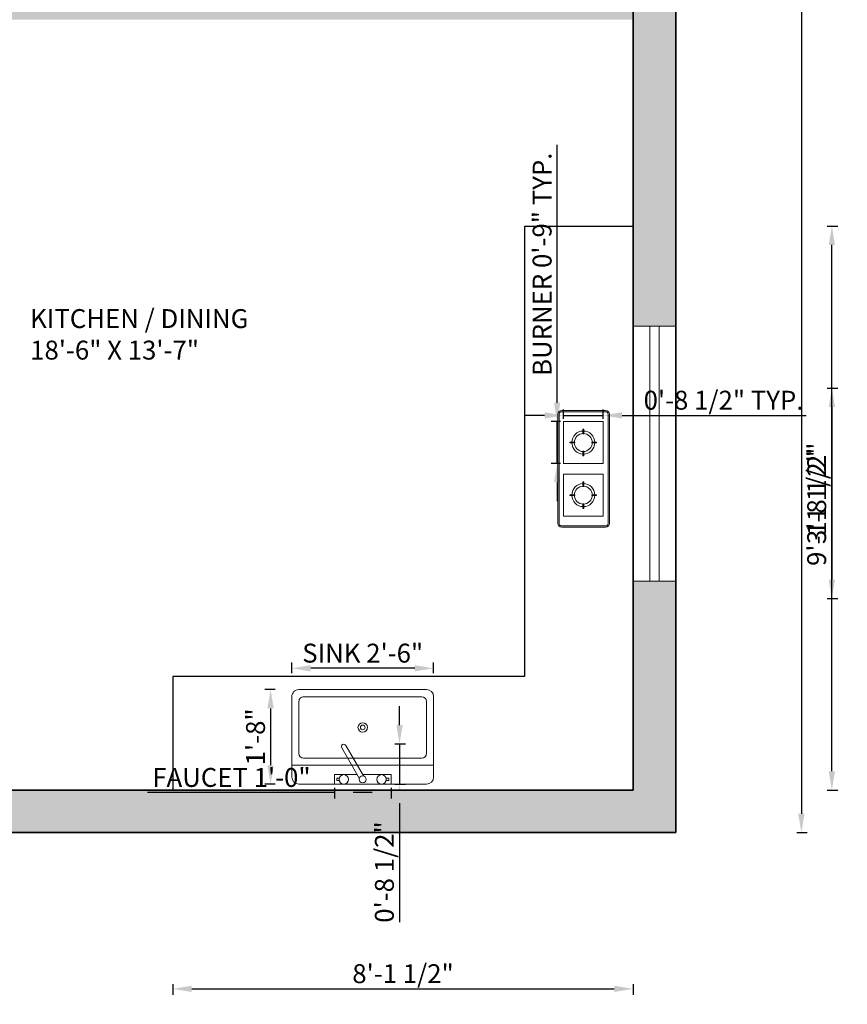
# Model space of a CAD drawing. Units: inches. Extents: x -91 to 518, y -600 to 105.
# Tile 2 of 4: x 343 to 518, y -600 to -391. Entities that reach past the tile are written whole.
import ezdxf

# ---------------------------------------------------------------- set-up
doc = ezdxf.new("R2010")
doc.units = ezdxf.units.IN
for name, color, linetype, lineweight in [('A-ANNO-DIMS', 2, 'Continuous', 18), ('A-AREA-IDEN', 7, 'Continuous', 18), ('A-EQPM', 8, 'Continuous', 18), ('A-FLOR-CASE', 9, 'Continuous', 25), ('A-FLOR-FIXT', 9, 'Continuous', 18), ('A-GLAZ', 6, 'Continuous', 18), ('A-WALL', 7, 'Continuous', 35), ('A-WALL-PATT', 251, 'Continuous', 13)]:
    doc.layers.add(name, color=color, linetype=linetype, lineweight=lineweight)
doc.styles.get("Standard").update_dxf_attribs({"font": 'arial.ttf'})
doc.dimstyles.new('ISO-25', dxfattribs={"dimtxt": 4, "dimasz": 4, "dimexe": 1.25, "dimexo": 0.625, "dimtad": 1, "dimlunit": 3, "dimtxsty": 'Standard', "dimcen": 2.5, "dimadec": 0, "dimazin": 0, "dimtfac": 1, "dimtmove": 0, "dimatfit": 3, "dimfxl": 1, "dimfxlon": 1, "dimarcsym": 0})

# ---------------------------------------------------------------- blocks, each defined once
blk = doc.blocks.new('Sink-single - 30 in top')
blk.add_line((-15, -3.999996000000001), (15, -3.999996000000001))
for points in [[(-13.5, 0), (13.5, 0)], [(-15, -18.499996), (-15, -1.500000000000001)], [(15, -1.500000000000001), (15, -18.499996)], [(-12.5, -5.499996000000001), (12.5, -5.499996000000001)], [(-13.5, -17.499996), (-13.5, -6.499996000000001)], [(13.5, -6.499996000000001), (13.5, -17.499996)], [(12.5, -18.499996), (-12.5, -18.499996)], [(13.5, -19.999996), (-13.5, -19.999996)]]:
    blk.add_lwpolyline(points)
for radius in [1, 0.5]:
    blk.add_circle((0, -11.999996), radius)
for centre, radius, start, end in [((-13.5, -1.500000000000001), 1.5, 90, 180), ((13.5, -1.500000000000001), 1.5, 0, 90), ((-12.5, -6.499996000000001), 1, 90, 180), ((12.5, -6.499996000000001), 1, 0, 90), ((-13.5, -18.499996), 1.5, 180, 270), ((-12.5, -17.499996), 1, 180, 270), ((12.5, -17.499996), 1, 270, 0), ((13.5, -18.499996), 1.5, 270, 0)]:
    blk.add_arc(centre, radius, start, end)
blk = doc.blocks.new('Faucet - kit sink top')
for p, q in [((-5.5, -0.75), (-5.5, -1.25)), ((-4.942779999999999, -0.75), (-5.5, -0.75)), ((-5.5, -1.25), (-4.942779999999999, -1.25)), ((-0.147750000000002, -1.744100000000003), (3.566980000000008, -8.178200000000002)), ((4.433010000000003, -7.678200000000003), (0.7182800000000072, -1.244100000000003)), ((4.942780000000006, -0.75), (5.5, -0.75)), ((5.5, -1.25), (4.942780000000006, -1.25)), ((5.5, -0.75), (5.5, -1.25))]:
    blk.add_line(p, q)
blk.add_lwpolyline([(-0.0058699999999945, -2), (-6, -2), (-6, 0), (6, 0), (6, -2), (1.151949999999999, -2)])
for centre, radius in [((-4, -1), 1), ((4, -1), 1), ((0, -1), 0.75)]:
    blk.add_circle(centre, radius)
blk.add_arc((4, -7.928200000000003), 0.5, 210, 30)
blk = doc.blocks.new('*D10')
at = {"layer": 'A-ANNO-DIMS', "color": 0, "lineweight": -2, "transparency": 16777216}
for p, q in [((507.1447856816575, 12.69286819609), (509.3947856816575, 12.69286819609)), ((508.1447856816574, 8.69286819609), (508.1447856816575, -559.3071318039102)), ((507.1447856816575, -563.3071318039102), (509.3947856816575, -563.3071318039102))]:
    blk.add_line(p, q, dxfattribs=at)
at = {"layer": 'A-ANNO-DIMS', "color": 0, "transparency": 16777216}
for points in [[(507.4781190149908, 8.692868196089998), (508.8114523483241, 8.69286819609), (508.1447856816574, 12.69286819609)], [(507.4781190149908, -559.3071318039102), (508.8114523483242, -559.3071318039102), (508.1447856816575, -563.3071318039102)]]:
    blk.add_solid(points, dxfattribs=at)
at = {"layer": 'Defpoints', "color": 0, "transparency": 16777216}
for p in [(481.543973026278, 12.69286819608999), (481.543973026278, -563.3071318039102), (508.1447856816575, -563.3071318039102)]:
    blk.add_point(p, dxfattribs=at)
at = {"layer": 'A-ANNO-DIMS', "color": 0, "transparency": 16777216, "insert": (505.4774937307706, -275.3071318039102), "char_height": 4, "attachment_point": 5, "rotation": 90}
blk.add_mtext("48'", dxfattribs=at)
blk = doc.blocks.new('WIN-54IN')
for p, q in [((-8.22649996337e-05, 5.500051768139757), (53.99991773500037, 5.500051768139757)), ((-8.22649996337e-05, 3.500051768139757), (53.99991773500037, 3.500051768139757))]:
    blk.add_line(p, q)
blk.add_lwpolyline([(-8.22649996337e-05, 9.000051768139757), (53.99991773500037, 9.000051768139757), (53.99991773500037, 5.17681397576e-05), (-8.22649996337e-05, 5.17681397576e-05)], close=True)
blk = doc.blocks.new('COOKTOP-BURNER')
for p, q in [((4.88062485715e-05, 0.0001151396265868), (4.88062485715e-05, 8.841393903745084)), ((4.88062485715e-05, 8.841393903745084), (8.420919979822145, 8.841393903745029)), ((8.420919979822145, 8.841393903745029), (8.420919979822145, 0.0001151396265868)), ((4.132223564928096, 6.231676937305905), (4.132223564928096, 7.249946376473928)), ((4.132223564928096, 7.249946376473928), (4.288745221142619, 7.249946376473928)), ((4.288745221142619, 7.249946376473928), (4.288745221142619, 6.231676937305905)), ((1.381292538244736, 4.342493693775679), (1.381292538244736, 4.499015349595936)), ((1.381292538244736, 4.499015349595936), (2.399561977612336, 4.499015349595936)), ((2.399561977612336, 4.342493693775679), (1.381292538244736, 4.342493693775679)), ((2.399561977612336, 4.499015349595936), (2.399561977612336, 4.342493693775679)), ((4.288745221142619, 6.231676937305905), (4.132223564928096, 6.231676937305905)), ((6.021406808459289, 4.342493693775679), (6.021406808459289, 4.499015349595936)), ((6.021406808459289, 4.499015349595936), (7.039676247826093, 4.499015349595936)), ((7.039676247826093, 4.342493693775679), (6.021406808459289, 4.342493693775679)), ((7.039676247826093, 4.499015349595936), (7.039676247826093, 4.342493693775679)), ((4.132223564928096, 2.609832106065709), (4.288745221142619, 2.609832106065709)), ((4.132223564928096, 1.591562666893594), (4.132223564928096, 2.609832106065709)), ((4.288745221142619, 2.609832106065709), (4.288745221142619, 1.591562666893594)), ((8.420919979822145, 0.0001151396265868), (4.88062485715e-05, 0.0001151396265868)), ((4.288745221142619, 1.591562666893594), (4.132223564928096, 1.591562666893594))]:
    blk.add_line(p, q)
for radius in [2.437545410726341, 1.897671920604797]:
    blk.add_circle((4.210484393035869, 4.420754521292622), radius)
blk = doc.blocks.new('*D26')
at = {"layer": 'A-ANNO-DIMS', "color": 0, "lineweight": -2, "transparency": 16777216}
for p, q in [((456.4408569914164, -472.3535935240309), (456.4408569914164, -417.7502510956544)), ((457.142048806034, -476.3535935240309), (455.1908569914165, -476.3535935240309)), ((456.4408569914164, -485.1948722881494), (456.4408569914164, -476.3535935240309)), ((457.142048806034, -485.1948722881494), (455.1908569914165, -485.1948722881494)), ((456.4408569914164, -489.1948722881494), (456.4408569914164, -493.1948722881494))]:
    blk.add_line(p, q, dxfattribs=at)
at = {"layer": 'A-ANNO-DIMS', "color": 0, "transparency": 16777216}
for points in [[(455.7741903247498, -472.3535935240309), (457.1075236580831, -472.3535935240309), (456.4408569914164, -476.3535935240309)], [(455.7741903247498, -489.1948722881494), (457.1075236580831, -489.1948722881494), (456.4408569914164, -485.1948722881494)]]:
    blk.add_solid(points, dxfattribs=at)
at = {"layer": 'Defpoints', "color": 0, "transparency": 16777216}
for p in [(456.4408569914164, -476.3535935240309), (457.767048806034, -476.3535935240309), (457.767048806034, -485.1948722881494)]:
    blk.add_point(p, dxfattribs=at)
at = {"layer": 'A-ANNO-DIMS', "color": 0, "transparency": 16777216, "insert": (453.7735650405295, -443.0519223098427), "char_height": 4, "attachment_point": 5, "rotation": 90}
blk.add_mtext('BURNER 0\'-9" TYP.', dxfattribs=at)
blk = doc.blocks.new('*D27')
at = {"layer": 'A-ANNO-DIMS', "color": 0, "lineweight": -2, "transparency": 16777216}
for p, q in [((457.7670488060338, -475.7285935240306), (457.7670488060338, -473.7774017094129)), ((466.1879199796074, -475.7285935240306), (466.1879199796074, -473.7774017094129)), ((453.7670488060338, -475.0274017094128), (449.7670488060338, -475.0274017094128)), ((457.7670488060338, -475.0274017094128), (466.1879199796074, -475.0274017094128)), ((470.1879199796074, -475.0274017094128), (509.1405120669199, -475.0274017094128))]:
    blk.add_line(p, q, dxfattribs=at)
at = {"layer": 'A-ANNO-DIMS', "color": 0, "transparency": 16777216}
for points in [[(453.7670488060338, -474.3607350427462), (453.7670488060338, -475.6940683760795), (457.7670488060338, -475.0274017094128)], [(470.1879199796074, -474.3607350427462), (470.1879199796074, -475.6940683760795), (466.1879199796074, -475.0274017094128)]]:
    blk.add_solid(points, dxfattribs=at)
at = {"layer": 'Defpoints', "color": 0, "transparency": 16777216}
for p in [(457.7670488060338, -476.3535935240307), (466.1879199796074, -475.0274017094128), (466.1879199796074, -476.3535935240307)]:
    blk.add_point(p, dxfattribs=at)
at = {"layer": 'A-ANNO-DIMS', "color": 0, "transparency": 16777216, "insert": (491.6642160232636, -472.334188885402), "char_height": 4, "attachment_point": 5}
blk.add_mtext('0\'-8 1/2" TYP.', dxfattribs=at)
blk = doc.blocks.new('*D28')
at = {"layer": 'A-ANNO-DIMS', "color": 0, "lineweight": -2, "transparency": 16777216}
for p, q in [((400.2823967097227, -529.5410858293926), (400.2823967097227, -527.2910858293926)), ((426.2823967097228, -528.5410858293926), (404.2823967097227, -528.5410858293926)), ((430.2823967097228, -529.5410858293926), (430.2823967097228, -527.2910858293926))]:
    blk.add_line(p, q, dxfattribs=at)
at = {"layer": 'A-ANNO-DIMS', "color": 0, "transparency": 16777216}
for points in [[(404.2823967097227, -527.874419162726), (404.2823967097227, -529.2077524960592), (400.2823967097227, -528.5410858293926)], [(426.2823967097228, -527.874419162726), (426.2823967097228, -529.2077524960592), (430.2823967097228, -528.5410858293926)]]:
    blk.add_solid(points, dxfattribs=at)
at = {"layer": 'Defpoints', "color": 0, "transparency": 16777216}
for p in [(400.2823967097227, -528.5410858293926), (400.2823967097227, -533.0410858293926), (430.2823967097228, -533.0410858293926)]:
    blk.add_point(p, dxfattribs=at)
at = {"layer": 'A-ANNO-DIMS', "color": 0, "transparency": 16777216, "insert": (415.2823967097227, -525.8478730053816), "char_height": 4, "attachment_point": 5}
blk.add_mtext('SINK 2\'-6"', dxfattribs=at)
blk = doc.blocks.new('*D29')
at = {"layer": 'A-ANNO-DIMS', "color": 0, "lineweight": -2, "transparency": 16777216}
for p, q in [((396.7823967097232, -533.0410858293928), (394.5323967097232, -533.0410858293928)), ((395.7823967097232, -537.0410858293928), (395.7823967097232, -549.0410818293929)), ((396.7823967097232, -553.0410818293929), (394.5323967097232, -553.0410818293929))]:
    blk.add_line(p, q, dxfattribs=at)
at = {"layer": 'A-ANNO-DIMS', "color": 0, "transparency": 16777216}
for points in [[(395.1157300430566, -537.0410858293928), (396.4490633763899, -537.0410858293928), (395.7823967097232, -533.0410858293928)], [(395.1157300430566, -549.0410818293929), (396.4490633763899, -549.0410818293929), (395.7823967097232, -553.0410818293929)]]:
    blk.add_solid(points, dxfattribs=at)
at = {"layer": 'Defpoints', "color": 0, "transparency": 16777216}
for p in [(400.282396709723, -533.0410858293928), (395.7823967097232, -553.0410818293929), (400.282396709723, -553.0410818293929)]:
    blk.add_point(p, dxfattribs=at)
at = {"layer": 'A-ANNO-DIMS', "color": 0, "transparency": 16777216, "insert": (393.1151047588362, -543.0410838293928), "char_height": 4, "attachment_point": 5, "rotation": 90}
blk.add_mtext('1\'-8"', dxfattribs=at)
blk = doc.blocks.new('*D30')
at = {"layer": 'A-ANNO-DIMS', "color": 0, "lineweight": -2, "transparency": 16777216}
for p, q in [((409.2823967097228, -553.8410818293925), (409.2823967097228, -556.0910818293925)), ((421.2823967097227, -553.8410818293925), (421.2823967097227, -556.0910818293925)), ((409.2823967097228, -554.8410818293925), (369.721346232233, -554.8410818293925)), ((417.2823967097228, -554.8410818293925), (413.2823967097228, -554.8410818293925))]:
    blk.add_line(p, q, dxfattribs=at)
at = {"layer": 'A-ANNO-DIMS', "color": 0, "transparency": 16777216}
for points in [[(413.2823967097228, -554.174415162726), (413.2823967097228, -555.5077484960592), (409.2823967097228, -554.8410818293925)], [(417.2823967097228, -554.174415162726), (417.2823967097228, -555.5077484960592), (421.2823967097227, -554.8410818293925)]]:
    blk.add_solid(points, dxfattribs=at)
at = {"layer": 'Defpoints', "color": 0, "transparency": 16777216}
for p in [(409.2823967097228, -553.0410818293926), (421.2823967097227, -553.0410818293926), (409.2823967097228, -554.8410818293925)]:
    blk.add_point(p, dxfattribs=at)
at = {"layer": 'A-ANNO-DIMS', "color": 0, "transparency": 16777216, "insert": (387.5018714709779, -552.1478690053815), "char_height": 4, "attachment_point": 5}
blk.add_mtext('FAUCET 1\'-0"', dxfattribs=at)
blk = doc.blocks.new('*D31')
at = {"layer": 'A-ANNO-DIMS', "color": 0, "lineweight": -2, "transparency": 16777216}
for p, q in [((423.0823967097232, -540.5417979400429), (423.0823967097232, -536.5417979400429)), ((422.0823967097232, -544.5417979400429), (424.3323967097232, -544.5417979400429)), ((423.0823967097232, -544.5417979400429), (423.0823967097232, -553.0410818293929)), ((422.0823967097232, -553.0410818293929), (424.3323967097232, -553.0410818293929)), ((423.0823967097232, -557.0410818293929), (423.0823967097232, -582.2446971090654))]:
    blk.add_line(p, q, dxfattribs=at)
at = {"layer": 'A-ANNO-DIMS', "color": 0, "transparency": 16777216}
for points in [[(422.4157300430565, -540.5417979400429), (423.7490633763899, -540.5417979400429), (423.0823967097232, -544.5417979400429)], [(422.4157300430565, -557.0410818293929), (423.7490633763899, -557.0410818293929), (423.0823967097232, -553.0410818293929)]]:
    blk.add_solid(points, dxfattribs=at)
at = {"layer": 'Defpoints', "color": 0, "transparency": 16777216}
for p in [(421.282396709723, -544.5417979400429), (421.282396709723, -553.0410818293929), (423.0823967097232, -553.0410818293929)]:
    blk.add_point(p, dxfattribs=at)
at = {"layer": 'A-ANNO-DIMS', "color": 0, "transparency": 16777216, "insert": (420.389183885712, -571.6428894692291), "char_height": 4, "attachment_point": 5, "rotation": 90}
blk.add_mtext('0\'-8 1/2"', dxfattribs=at)
blk = doc.blocks.new('*D37')
at = {"layer": 'A-ANNO-DIMS', "color": 0, "lineweight": -2, "transparency": 16777216}
for p, q in [((-80.98865400000005, -530.3071320000003), (-83.23865400000007, -530.3071320000003)), ((-81.98865400000005, -534.3071320000003), (-81.98865400000004, -550.3071320000003)), ((-80.98865400000005, -554.3071320000003), (-83.23865400000005, -554.3071320000003))]:
    blk.add_line(p, q, dxfattribs=at)
at = {"layer": 'A-ANNO-DIMS', "color": 0, "transparency": 16777216}
for points in [[(-82.65532066666673, -534.3071320000003), (-81.32198733333337, -534.3071320000003), (-81.98865400000005, -530.3071320000003)], [(-82.6553206666667, -550.3071320000003), (-81.32198733333337, -550.3071320000003), (-81.98865400000004, -554.3071320000003)]]:
    blk.add_solid(points, dxfattribs=at)
at = {"layer": 'Defpoints', "color": 0, "transparency": 16777216}
for p in [(375.0870760000001, -530.3071320000003), (-81.98865400000004, -554.3071320000003), (375.0870760000001, -554.3071320000003)]:
    blk.add_point(p, dxfattribs=at)
at = {"layer": 'A-ANNO-DIMS', "color": 0, "transparency": 16777216, "insert": (-84.65594595088695, -542.3071320000003), "char_height": 4, "attachment_point": 5, "rotation": 90}
blk.add_mtext('2\'-0"', dxfattribs=at)
blk = doc.blocks.new('*D38')
at = {"layer": 'A-ANNO-DIMS', "color": 0, "lineweight": -2, "transparency": 16777216}
for p, q in [((449.608002, 95.58768199999997), (449.608002, 97.83768199999997)), ((453.608002, 96.587682), (468.543973, 96.587682)), ((472.543973, 95.58768199999997), (472.543973, 97.83768199999997))]:
    blk.add_line(p, q, dxfattribs=at)
at = {"layer": 'A-ANNO-DIMS', "color": 0, "transparency": 16777216}
for points in [[(453.608002, 97.25434866666667), (453.608002, 95.92101533333332), (449.608002, 96.587682)], [(468.543973, 97.25434866666667), (468.543973, 95.92101533333332), (472.543973, 96.587682)]]:
    blk.add_solid(points, dxfattribs=at)
at = {"layer": 'Defpoints', "color": 0, "transparency": 16777216}
for p in [(472.543973, 96.587682), (449.6080019999999, -434.9571809999999), (472.5439729999999, -434.9571809999999)]:
    blk.add_point(p, dxfattribs=at)
at = {"layer": 'A-ANNO-DIMS', "color": 0, "transparency": 16777216, "insert": (461.0759875, 99.2208675388813), "char_height": 4, "attachment_point": 5}
blk.add_mtext('1\'-11"', dxfattribs=at)
blk = doc.blocks.new('*D39')
at = {"layer": 'A-ANNO-DIMS', "color": 0, "lineweight": -2, "transparency": 16777216}
for p, q in [((375.087076, -595.357132), (375.087076, -597.6071319999999)), ((472.5439729999999, -595.357132), (472.5439729999999, -597.6071319999999)), ((379.087076, -596.3571319999999), (468.5439729999999, -596.3571319999999))]:
    blk.add_line(p, q, dxfattribs=at)
at = {"layer": 'A-ANNO-DIMS', "color": 0, "transparency": 16777216}
for points in [[(379.087076, -595.6904653333333), (379.087076, -597.0237986666666), (375.087076, -596.3571319999999)], [(468.5439729999999, -595.6904653333333), (468.5439729999999, -597.0237986666666), (472.5439729999999, -596.3571319999999)]]:
    blk.add_solid(points, dxfattribs=at)
at = {"layer": 'Defpoints', "color": 0, "transparency": 16777216}
for p in [(375.087076, -554.307132), (472.5439729999999, -554.307132), (472.5439729999999, -596.3571319999999)]:
    blk.add_point(p, dxfattribs=at)
at = {"layer": 'A-ANNO-DIMS', "color": 0, "transparency": 16777216, "insert": (423.8155245, -593.6639191759891), "char_height": 4, "attachment_point": 5}
blk.add_mtext('8\'-1 1/2"', dxfattribs=at)
blk = doc.blocks.new('*D40')
at = {"layer": 'A-ANNO-DIMS', "color": 0, "lineweight": -2, "transparency": 16777216}
for p, q in [((513.5939730000003, -434.9571810000002), (515.8439730000003, -434.9571810000002)), ((514.5939730000003, -550.3071320000003), (514.5939730000003, -438.9571810000002)), ((513.5939730000003, -554.3071320000003), (515.8439730000003, -554.3071320000003))]:
    blk.add_line(p, q, dxfattribs=at)
at = {"layer": 'A-ANNO-DIMS', "color": 0, "transparency": 16777216}
for points in [[(513.9273063333338, -438.9571810000002), (515.260639666667, -438.9571810000002), (514.5939730000003, -434.9571810000002)], [(513.9273063333338, -550.3071320000003), (515.260639666667, -550.3071320000003), (514.5939730000003, -554.3071320000003)]]:
    blk.add_solid(points, dxfattribs=at)
at = {"layer": 'Defpoints', "color": 0, "transparency": 16777216}
for p in [(472.5439730000002, -434.9571810000002), (514.5939730000003, -434.9571810000002), (472.5439730000002, -554.3071320000003)]:
    blk.add_point(p, dxfattribs=at)
at = {"layer": 'A-ANNO-DIMS', "color": 0, "transparency": 16777216, "insert": (511.9007601759892, -494.6321565000003), "char_height": 4, "attachment_point": 5, "rotation": 90}
blk.add_mtext('9\'-11 1/2"', dxfattribs=at)
blk = doc.blocks.new('*D50')
at = {"layer": 'A-ANNO-DIMS', "color": 0, "lineweight": -2, "transparency": 16777216}
for p, q in [((-80.9886540000001, -391.3071320000003), (-83.2386540000001, -391.3071320000003)), ((-81.98865400000007, -395.3071320000003), (-81.98865400000005, -452.1362110000002)), ((-80.98865400000008, -456.1362110000002), (-83.23865400000007, -456.1362110000002))]:
    blk.add_line(p, q, dxfattribs=at)
at = {"layer": 'A-ANNO-DIMS', "color": 0, "transparency": 16777216}
for points in [[(-82.65532066666674, -395.3071320000003), (-81.3219873333334, -395.3071320000003), (-81.98865400000007, -391.3071320000003)], [(-82.65532066666673, -452.1362110000002), (-81.32198733333337, -452.1362110000002), (-81.98865400000005, -456.1362110000002)]]:
    blk.add_solid(points, dxfattribs=at)
at = {"layer": 'Defpoints', "color": 0, "transparency": 16777216}
for p in [(472.5439730000002, -391.3071320000002), (-81.98865400000005, -456.1362110000002), (472.5439730000002, -456.1362110000002)]:
    blk.add_point(p, dxfattribs=at)
at = {"layer": 'A-ANNO-DIMS', "color": 0, "transparency": 16777216, "insert": (-84.64776041200562, -423.7216715000001), "char_height": 4, "attachment_point": 5, "rotation": 90}
blk.add_mtext('5\'-5"', dxfattribs=at)
blk = doc.blocks.new('*D55')
at = {"layer": 'A-ANNO-DIMS', "color": 0, "lineweight": -2, "transparency": 16777216}
for p, q in [((513.5939730000003, -469.2346910000002), (515.8439730000003, -469.2346910000002)), ((514.5939730000003, -473.2346910000002), (514.5939730000003, -509.7744600000002)), ((513.5939730000003, -513.7744600000002), (515.8439730000003, -513.7744600000002))]:
    blk.add_line(p, q, dxfattribs=at)
at = {"layer": 'A-ANNO-DIMS', "color": 0, "transparency": 16777216}
for points in [[(513.9273063333338, -473.2346910000002), (515.260639666667, -473.2346910000002), (514.5939730000003, -469.2346910000002)], [(513.9273063333338, -509.7744600000002), (515.260639666667, -509.7744600000002), (514.5939730000003, -513.7744600000002)]]:
    blk.add_solid(points, dxfattribs=at)
at = {"layer": 'Defpoints', "color": 0, "transparency": 16777216}
for p in [(296.0378580000001, -469.2346910000002), (296.0378580000001, -513.7744600000002), (514.5939730000003, -513.7744600000002)]:
    blk.add_point(p, dxfattribs=at)
at = {"layer": 'A-ANNO-DIMS', "color": 0, "transparency": 16777216, "insert": (511.8993959195091, -491.5045755000003), "char_height": 4, "attachment_point": 5, "rotation": 90}
blk.add_mtext('3\'-8 1/2"', dxfattribs=at)
blk = doc.blocks.new('*D58')
at = {"layer": 'A-ANNO-DIMS', "color": 0, "lineweight": -2, "transparency": 16777216}
for p, q in [((375.0870760000001, 95.58768199999997), (375.0870760000001, 97.83768199999997)), ((379.0870760000001, 96.587682), (396.7217370000001, 96.587682)), ((400.7217370000001, 95.58768199999997), (400.7217370000001, 97.83768199999997))]:
    blk.add_line(p, q, dxfattribs=at)
at = {"layer": 'A-ANNO-DIMS', "color": 0, "transparency": 16777216}
for points in [[(379.0870760000001, 97.25434866666667), (379.0870760000001, 95.92101533333332), (375.0870760000001, 96.587682)], [(396.7217370000001, 97.25434866666667), (396.7217370000001, 95.92101533333332), (400.7217370000001, 96.587682)]]:
    blk.add_solid(points, dxfattribs=at)
at = {"layer": 'Defpoints', "color": 0, "transparency": 16777216}
for p in [(400.7217370000001, 96.587682), (375.087076, -530.3071319999999), (400.721737, -533.4804259999999)]:
    blk.add_point(p, dxfattribs=at)
at = {"layer": 'A-ANNO-DIMS', "color": 0, "transparency": 16777216, "insert": (387.9044065, 99.28089482401091), "char_height": 4, "attachment_point": 5}
blk.add_mtext('2\'-1 1/2"', dxfattribs=at)

msp = doc.modelspace()

# ---------------------------------------------------------------- hatches: boundary and pattern name
at = {"layer": 'A-WALL-PATT'}
h = msp.add_hatch(color=256, dxfattribs=at)
h.dxf.hatch_style = 1
h.paths.add_polyline_path([(10.54397302627791, 3.69286819609001), (34.46210501665792, 3.692868196090003), (34.46210501665792, 12.69286819609001), (1.54397302627791, 12.69286819609001), (1.54397302627791, -180.8777568066362), (10.54397302627791, -180.8777568066362)])
h.paths.add_polyline_path([(46.54397302627785, -92.30713180391), (10.54397302627791, -92.30713180390997), (10.54397302627791, -98.30713180391), (46.54397302627785, -98.30713180391001)])
h.paths.add_polyline_path([(130.3809177350003, 12.69286819608999), (52.46210501665791, 12.69286819608999), (52.46210501665792, 3.692868196090003), (82.54397302627785, 3.692868196090003), (88.54397302627785, 3.692868196090003), (130.3809177350004, 3.692868196090003)])
h.paths.add_polyline_path([(88.5439730262779, 3.692868196089996), (82.54397302627792, 3.692868196089996), (82.54397302627792, -92.30713180390997), (76.54397302627785, -92.30713180391001), (76.54397302627785, -94.37012392989423), (76.54397302627785, -98.30713180391001), (82.5439730262779, -98.30713180391), (82.5439730262779, -106.0567926816102), (85.5222416603892, -106.0567926816102), (88.54397302627791, -106.0567926816102)])
h.paths.add_polyline_path([(250.5439730262778, -146.30713180391), (245.7716552283821, -146.30713180391), (244.5439730262779, -146.30713180391), (244.5439730262779, -152.30713180391), (88.54397302627791, -152.3071318039099), (88.54397302627791, -141.7441975357105), (85.71753115439951, -141.7441975357105), (82.54397302627792, -141.7441975357105), (82.54397302627792, -152.3071318039099), (10.54397302627791, -152.3071318039099), (10.54397302627791, -158.30713180391), (88.54397302627785, -158.30713180391), (118.5439730262778, -158.30713180391), (118.5439730262778, -164.30713180391), (120.6069651522621, -164.30713180391), (124.5439730262778, -164.30713180391), (124.5439730262778, -158.3071318039099), (244.5439730262779, -158.30713180391), (244.5439730262779, -164.30713180391), (250.5439730262779, -164.30713180391)])
h.paths.add_polyline_path([(274.3406872340411, 12.69286819609), (184.3809177350003, 12.69286819609), (184.3809177350003, 3.692868196089996), (244.5439730262779, 3.692868196089996), (250.5439730262779, 3.692868196089996), (274.3406872340411, 3.692868196090003)])
h.paths.add_polyline_path([(250.5439730262779, 3.692868196090003), (244.5439730262779, 3.692868196089989), (244.5439730262779, -110.30713180391), (250.5439730262779, -110.30713180391), (250.5439730262779, -98.30713180391), (310.5439730262779, -98.30713180391001), (310.5439730262779, -110.30713180391), (316.5439730262779, -110.30713180391), (316.5439730262779, -86.51662232277216), (312.6069651522621, -86.51662232277216), (310.5439730262779, -86.51662232277216), (310.543973026278, -92.30713180391001), (250.5439730262779, -92.30713180390997)])
h.paths.add_polyline_path([(481.5439730262779, 12.69286819608999), (292.3406872340411, 12.69286819609), (292.3406872340411, 3.692868196089989), (310.5439730262779, 3.692868196089996), (316.5439730262779, 3.692868196089996), (472.5439730262779, 3.692868196089989), (472.5439730262778, -34.12947996685534), (481.5439730262779, -34.12947996685534)])
h.paths.add_polyline_path([(316.5439730262779, 3.692868196090003), (310.5439730262779, 3.692868196089996), (310.5439730262779, -56.51662232277216), (316.5439730262779, -56.51662232277216)], flags=17)
h.paths.add_polyline_path([(481.543973026278, -88.12947996685536), (472.5439730262779, -88.12947996685536), (472.5439730262779, -189.4514204144393), (481.5439730262779, -189.4514204144393)])
h.paths.add_polyline_path([(472.5439730262779, -152.30713180391), (316.5439730262779, -152.30713180391), (316.5439730262779, -146.30713180391), (315.3190113957458, -146.30713180391), (310.5439730262779, -146.30713180391), (310.5439730262779, -260.30713180391), (316.543973026278, -260.30713180391), (316.5439730262779, -158.30713180391), (472.5439730262778, -158.30713180391)])
h.paths.add_polyline_path([(481.5439730262779, -243.4514204144393), (472.5439730262778, -243.4514204144393), (472.5439730262779, -308.30713180391), (472.5439730262779, -332.5934456982646), (481.5439730262779, -332.5934456982646)])
h.paths.add_polyline_path([(472.543973026278, -302.30713180391), (316.5439730262779, -302.30713180391), (316.543973026278, -296.30713180391), (315.3223312342462, -296.30713180391), (310.5439730262779, -296.30713180391), (310.5439730262779, -308.3071318039099), (472.543973026278, -308.3071318039101)])
h.paths.add_polyline_path([(481.543973026278, -366.5934456982646), (472.5439730262779, -366.5934456982645), (472.5439730262779, -385.30713180391), (472.5439730262779, -456.1362109337742), (481.5439730262779, -456.1362109337742)])
h.paths.add_polyline_path([(472.543973026278, -385.3071318039099), (310.543973026278, -385.30713180391), (310.5439730262779, -391.30713180391), (472.543973026278, -391.30713180391)])
h.paths.add_polyline_path([(481.543973026278, -510.1362109337741), (472.5439730262779, -510.1362109337741), (472.5439730262778, -554.30713180391), (323.1846508389144, -554.30713180391), (323.1846508389144, -563.30713180391), (481.5439730262779, -563.30713180391)])
h.paths.add_polyline_path([(250.5439730262778, -384.7238270396974), (229.6450614403802, -384.7238270396974), (229.6450614403802, -393.7238270396975), (241.5439730262779, -393.7238270396974), (241.5439730262779, -563.30713180391), (269.1846508389144, -563.30713180391), (269.1846508389144, -554.30713180391), (250.5439730262779, -554.30713180391)])
h.paths.add_polyline_path([(195.6450614403802, -384.7238270396974), (133.7004703433376, -384.7238270396974), (133.7004703433376, -393.7238270396974), (195.6450614403802, -393.7238270396975)])
h.paths.add_polyline_path([(99.70047034333766, -384.7238270396975), (61.54397302627785, -384.7238270396975), (61.54397302627785, -391.562077029412), (61.33486888165797, -393.7238270396973), (77.04231968784188, -393.7238270396973), (99.70047034333767, -393.7238270396973)])
h.paths.add_polyline_path([(10.54397302627791, -264.0141460456657), (1.54397302627791, -264.0141460456657), (1.543973026277911, -330.0475231407777), (10.54397302627791, -330.0475231407777)])
h.paths.add_polyline_path([(10.54397302627791, -198.8777568066362), (1.54397302627791, -198.8777568066361), (1.543973026277911, -230.0141460456657), (10.54397302627791, -230.0141460456657)])
h.paths.add_polyline_path([(208.5439730262779, -218.30713180391), (124.5439730262779, -218.30713180391), (124.5439730262778, -194.30713180391), (118.5439730262778, -194.30713180391), (118.5439730262778, -218.30713180391), (10.54397302627791, -218.30713180391), (10.54397302627791, -224.30713180391), (118.5439730262778, -224.30713180391), (124.5439730262778, -224.30713180391), (208.5439730262778, -224.30713180391)])
h.paths.add_polyline_path([(250.5439730262778, -194.30713180391), (244.5439730262779, -194.30713180391), (244.5439730262779, -218.30713180391), (238.5439730262779, -218.30713180391), (238.5439730262779, -224.30713180391), (244.5439730262779, -224.30713180391), (244.5439730262778, -384.7238270396974), (250.5439730262779, -384.7238270396975)])

# ---------------------------------------------------------------- linework, layer by layer
at = {"layer": 'A-EQPM'}
for p, q in [((456.6112456040062, -474.7947941462856), (456.6112456040062, -497.8806842387522)), ((456.8811823489253, -474.7947941462856), (456.8811823489253, -497.8806842387522)), ((466.6990305807217, -473.9849839111339), (457.4210558391569, -473.9849839111339)), ((466.6990305807217, -474.2549206556629), (457.4210558391569, -474.2549206556629)), ((467.2389040709532, -497.8806842387523), (467.2389040709532, -474.7947941462856)), ((467.5088408158724, -497.8806842387523), (467.5088408158724, -474.7947941462856)), ((457.4210558391569, -498.4205577285885), (466.6990305807217, -498.4205577285886)), ((457.4210558391569, -498.6904944738999), (466.6990305807217, -498.6904944738999))]:
    msp.add_line(p, q, dxfattribs=at)
for centre, radius, start, end in [((457.4210558391569, -474.7947941462856), 0.8098102351823118, 90, 180), ((457.4210558391569, -474.7947941462856), 0.5398734901215415, 90, 180), ((466.6990305807217, -474.7947941462856), 0.8098102351823118, 0, 90), ((466.6990305807217, -474.7947941462856), 0.5398734901215415, 0, 90), ((457.4210558391569, -497.8806842387522), 0.8098102351823118, 180, 270), ((457.4210558391569, -497.8806842387522), 0.5398734901215415, 180, 270), ((466.6990305807217, -497.8806842387523), 0.5398734901215415, 270, 0), ((466.6990305807217, -497.8806842387523), 0.8098102351823118, 270, 0)]:
    msp.add_arc(centre, radius, start, end, dxfattribs=at)
at = {"layer": 'A-FLOR-CASE'}
for p, q in [((449.6080016436526, -530.30713180391), (449.6080016436526, -434.9571811499745)), ((449.6080016436526, -434.9571811499745), (472.5439730262778, -434.9571811499745)), ((449.6080016436526, -530.30713180391), (375.0870761066308, -530.30713180391)), ((375.0870761066308, -530.30713180391), (375.0870761066308, -554.30713180391))]:
    msp.add_line(p, q, dxfattribs=at)
at = {"layer": 'A-WALL'}
for p, q in [((481.5439730262779, 12.69286819608999), (481.5439730262779, -563.30713180391)), ((472.5439730262779, -385.30713180391), (472.5439730262778, -554.30713180391)), ((472.5439730262778, -554.30713180391), (250.5439730262779, -554.30713180391)), ((481.5439730262779, -563.30713180391), (1.54397302627791, -563.30713180391))]:
    msp.add_line(p, q, dxfattribs=at)

# ---------------------------------------------------------------- block references
at = {"layer": 'A-EQPM'}
for p in [(457.7669999997853, -485.1949874277758), (457.767, -496.3219999999999)]:
    msp.add_blockref('COOKTOP-BURNER', p, dxfattribs=at)
at = {"layer": 'A-FLOR-FIXT', "rotation": 180}
for name in ['Sink-single - 30 in top', 'Faucet - kit sink top']:
    msp.add_blockref(name, (415.2823967097228, -553.0410818293926), dxfattribs=at)
at = {"layer": 'A-GLAZ', "rotation": 269.9999999999999}
msp.add_blockref('WIN-54IN', (472.5439212581381, -456.1362931987737), dxfattribs=at)

# ---------------------------------------------------------------- texts
at = {"layer": 'A-AREA-IDEN', "insert": (344.8940335818006, -452.5485655981147), "char_height": 4, "attachment_point": 1}
msp.add_mtext_dynamic_manual_height_columns('KITCHEN / DINING\\P18\'-6" X 13\'-7"', width=64.60262232678906, gutter_width=12.5, heights=[0], dxfattribs=at)

# ---------------------------------------------------------------- dimensions: what is measured, and where the dimension line sits
at = {"layer": 'A-ANNO-DIMS'}
for base, p1, p2, picture, middle in [((400.7217370000001, 96.587682), (375.087076, -530.3071319999999), (400.721737, -533.4804259999999), '*D58', (387.9044065, 99.28089482401091)), ((472.543973, 96.587682), (449.6080019999999, -434.9571809999999), (472.5439729999999, -434.9571809999999), '*D38', (461.0759875, 99.2208675388813)), ((472.5439729999999, -596.3571319999999), (375.087076, -554.307132), (472.5439729999999, -554.307132), '*D39', (423.8155245, -593.6639191759891))]:
    dim = msp.add_linear_dim(base=base, p1=p1, p2=p2, dimstyle='ISO-25', override={"dimdec": 1, "dimlfac": 1, "dimrnd": 0, "dimzin": 1, "dimdsep": 46, "dimlunit": 4, "dimfrac": 2}, dxfattribs=at)
    dim.commit()
    dim.dimension.update_dxf_attribs({"geometry": picture, "text_midpoint": middle})
for base, p1, p2, angle, override, picture, middle in [((508.1447856816575, -563.3071318039102), (481.5439730262778, 12.69286819608999), (481.5439730262778, -563.30713180391), 90, {"dimclrd": 0, "dimclre": 0, "dimclrt": 0}, '*D10', (505.4774937307706, -275.3071318039102)), ((-81.98865400000005, -456.1362110000002), (472.5439729999999, -391.307132), (472.5439729999999, -456.136211), 90, {"dimdec": 1, "dimlfac": 1, "dimrnd": 0, "dimzin": 1, "dimdsep": 46, "dimlunit": 4, "dimfrac": 2}, '*D50', (-84.64776041200562, -423.7216715000001)), ((514.5939730000003, -434.9571810000002), (472.5439729999999, -554.307132), (472.5439729999999, -434.9571809999999), 90, {"dimdec": 1, "dimlfac": 1, "dimrnd": 0, "dimzin": 1, "dimdsep": 46, "dimlunit": 4, "dimfrac": 2}, '*D40', (511.9007601759892, -494.6321565000003)), ((514.5939730000003, -513.7744600000002), (296.037858, -469.234691), (296.037858, -513.7744599999999), 90, {"dimdec": 1, "dimlfac": 1, "dimrnd": 0, "dimzin": 1, "dimdsep": 46, "dimlunit": 4, "dimfrac": 2}, '*D55', (511.8993959195091, -491.5045755000003)), ((-81.98865400000004, -554.3071320000003), (375.087076, -530.3071319999999), (375.087076, -554.307132), 90, {"dimdec": 1, "dimlfac": 1, "dimrnd": 0, "dimzin": 1, "dimdsep": 46, "dimlunit": 4, "dimfrac": 2}, '*D37', (-84.65594595088695, -542.3071320000003)), ((395.7823967097232, -553.0410818293929), (400.2823967097227, -533.0410858293926), (400.2823967097227, -553.0410818293926), 270, {"dimdec": 1, "dimlfac": 1, "dimrnd": 0, "dimzin": 1, "dimdsep": 46, "dimlunit": 4, "dimfrac": 2}, '*D29', (393.1151047588362, -543.0410838293928)), ((423.0823967097232, -553.0410818293929), (421.2823967097227, -544.5417979400426), (421.2823967097227, -553.0410818293926), 270, {"dimdec": 1, "dimlfac": 1, "dimrnd": 0, "dimzin": 1, "dimdsep": 46, "dimlunit": 4, "dimfrac": 2}, '*D31', (420.389183885712, -571.6428894692291))]:
    dim = msp.add_linear_dim(base=base, p1=p1, p2=p2, angle=angle, dimstyle='ISO-25', override=override, dxfattribs=at)
    dim.commit()
    dim.dimension.update_dxf_attribs({"geometry": picture, "text_midpoint": middle})
for base, p1, p2, angle, text, picture, middle in [((456.4408569914164, -476.3535935240309), (457.7670488060338, -485.1948722881492), (457.7670488060338, -476.3535935240307), 90, 'BURNER <> TYP.', '*D26', (453.7735650405295, -443.0519223098427)), ((400.2823967097227, -528.5410858293926), (430.2823967097228, -533.0410858293926), (400.2823967097227, -533.0410858293926), 180, 'SINK <>', '*D28', (415.2823967097227, -525.8478730053816)), ((409.2823967097228, -554.8410818293925), (421.2823967097227, -553.0410818293926), (409.2823967097228, -553.0410818293926), 180, 'FAUCET <>', '*D30', (387.5018714709779, -552.1478690053815))]:
    dim = msp.add_linear_dim(base=base, p1=p1, p2=p2, angle=angle, text=text, dimstyle='ISO-25', override={"dimdec": 1, "dimlfac": 1, "dimrnd": 0, "dimzin": 1, "dimdsep": 46, "dimlunit": 4, "dimfrac": 2}, dxfattribs=at)
    dim.commit()
    dim.dimension.update_dxf_attribs({"geometry": picture, "text_midpoint": middle})
dim = msp.add_linear_dim(base=(466.1879199796074, -475.0274017094128), p1=(457.7670488060338, -476.3535935240307), p2=(466.1879199796074, -476.3535935240307), text='<> TYP.', dimstyle='ISO-25', override={"dimdec": 1, "dimlfac": 1, "dimrnd": 0, "dimzin": 1, "dimdsep": 46, "dimlunit": 4, "dimfrac": 2}, dxfattribs=at)
dim.commit()
dim.dimension.update_dxf_attribs({"geometry": '*D27', "text_midpoint": (491.6642160232636, -472.334188885402)})

doc.saveas('drawing.dxf')
